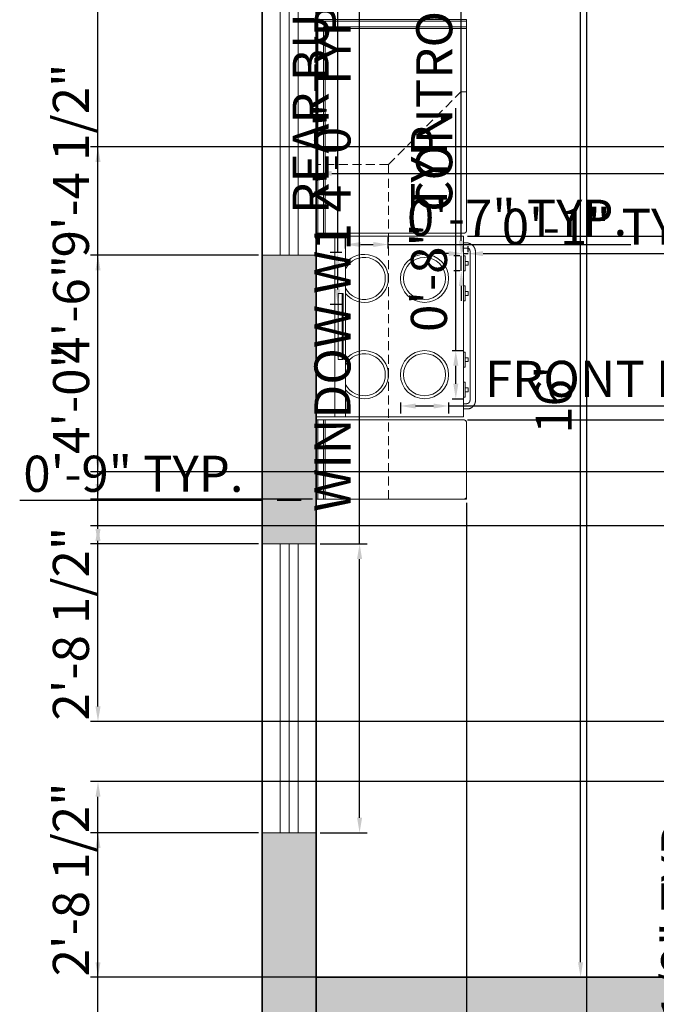
# Model space of a CAD drawing. Units: inches. Extents: x -40 to 424, y -33 to 568.
# Tile 4 of 8: x -40 to 66, y 275 to 438. Entities that reach past the tile are written whole.
import ezdxf

# ---------------------------------------------------------------- set-up
doc = ezdxf.new("R2010")
doc.units = ezdxf.units.IN
doc.linetypes.add('DASHED', pattern=[0.75, 0.5, -0.25])
for name, color, linetype, lineweight in [('A-ANNO-DIMS', 7, 'Continuous', 18), ('A-EQPM', 7, 'Continuous', 13), ('A-FLOR-CASE', 7, 'Continuous', 18), ('A-FLOR-CASE-HIDN', 7, 'DASHED', 13), ('A-GLAZ', 7, 'Continuous', 18), ('A-WALL-PATT', 30, 'Continuous', 13), ('wall', 7, 'Continuous', 35)]:
    doc.layers.add(name, color=color, linetype=linetype, lineweight=lineweight)
doc.styles.get("Standard").update_dxf_attribs({"font": 'arial.ttf'})
doc.dimstyles.new('ISO-25', dxfattribs={"dimtxt": 6, "dimasz": 2.5, "dimexe": 1.25, "dimexo": 0.625, "dimtad": 1, "dimdec": 1, "dimlunit": 3, "dimtxsty": 'Standard', "dimcen": 2.5, "dimadec": 0, "dimazin": 0, "dimtfac": 1, "dimtdec": 1, "dimtmove": 0, "dimatfit": 3, "dimfxl": 1, "dimarcsym": 0})

# ---------------------------------------------------------------- blocks, each defined once
blk = doc.blocks.new('*D27')
at = {"layer": 'A-ANNO-DIMS', "color": 0, "lineweight": -2, "transparency": 16777216}
for p, q in [((52.32, 471), (51.7, 471)), ((52.95, 281.5), (52.95, 468.5)), ((53.57, 279), (54.2, 279))]:
    blk.add_line(p, q, dxfattribs=at)
at = {"layer": 'A-ANNO-DIMS', "color": 0, "transparency": 16777216}
for points in [[(52.53, 468.5), (53.36, 468.5), (52.95, 471)], [(52.53, 281.5), (53.36, 281.5), (52.95, 279)]]:
    blk.add_solid(points, dxfattribs=at)
at = {"layer": 'Defpoints', "color": 0, "transparency": 16777216}
for p in [(52.95, 471), (52.95, 471), (52.95, 279)]:
    blk.add_point(p, dxfattribs=at)
at = {"layer": 'A-ANNO-DIMS', "color": 0, "transparency": 16777216, "insert": (49.26, 375), "char_height": 6, "attachment_point": 5, "rotation": 90}
blk.add_mtext("16'", dxfattribs=at)
blk = doc.blocks.new('*D28')
at = {"layer": 'A-ANNO-DIMS', "color": 0, "lineweight": -2, "transparency": 16777216}
for p, q in [((9.08, 457.74), (9.08, 411.34)), ((165, 457.74), (165, 411.34)), ((11.58, 412.59), (162.5, 412.59))]:
    blk.add_line(p, q, dxfattribs=at)
at = {"layer": 'A-ANNO-DIMS', "color": 0, "transparency": 16777216}
for points in [[(11.58, 413.01), (11.58, 412.18), (9.08, 412.59)], [(162.5, 413.01), (162.5, 412.18), (165, 412.59)]]:
    blk.add_solid(points, dxfattribs=at)
at = {"layer": 'Defpoints', "color": 0, "transparency": 16777216}
for p in [(9.08, 458.36), (165, 458.36), (165, 412.59)]:
    blk.add_point(p, dxfattribs=at)
at = {"layer": 'A-ANNO-DIMS', "color": 0, "transparency": 16777216, "insert": (87.04, 416.28), "char_height": 6, "attachment_point": 5}
blk.add_mtext('12\'-11.9"', dxfattribs=at)
blk = doc.blocks.new('WIN-48IN')
for p, q in [((0, 0), (0, 9)), ((48, 0), (48, 9)), ((0, 6), (48, 6)), ((0, 4.5), (48, 4.5)), ((0, 3), (48, 3))]:
    blk.add_line(p, q)
blk = doc.blocks.new('RANGE-CONTROL')
for p, q in [((0, 2.5), (0.25, 2.5)), ((0, 2.5), (0, 2.46)), ((0, 2.46), (0, 2.33)), ((0, 2.33), (0, 2.13)), ((0, 2.13), (0, 1.87)), ((0, 1.87), (0, 1.57)), ((0.25, 2.46), (0.25, 2.5)), ((0.25, 2.33), (0.25, 2.46)), ((0.25, 2.13), (0.25, 2.33)), ((0.25, 2.13), (0.25, 1.87)), ((0.25, 1.57), (0.25, 1.87)), ((0, 1.57), (0, 1.25)), ((0, 1.25), (0, 0.93)), ((0, 0.93), (0, 0.62)), ((0, 0.62), (0, 0.37)), ((0, 0.37), (0, 0.17)), ((0, 0.17), (0, 0.04)), ((0, 0.04), (0, 0)), ((0.25, 1.57), (0.25, 1.25)), ((0.25, 1.57), (0.75, 1.57)), ((0.25, 1.25), (0.25, 0.93)), ((0.25, 0.93), (0.25, 0.62)), ((0.25, 0.93), (0.75, 0.93)), ((0.25, 0.62), (0.25, 0.37)), ((0.25, 0.37), (0.25, 0.17)), ((0.25, 0.17), (0.25, 0.04)), ((0.25, 0.04), (0.25, 0)), ((0.75, 0.93), (0.75, 1.57)), ((0, 0), (0.25, 0))]:
    blk.add_line(p, q)
blk = doc.blocks.new('RANGE-BURNER-FRONT')
for radius in [4, 3.5]:
    blk.add_circle((4, 4), radius)
blk = doc.blocks.new('RANGE-BURNER-REAR')
for radius, start, end in [(4, 218.9563, 141.0437), (3.5, 207.2878, 152.7122)]:
    blk.add_arc((3.11, 4), radius, start, end)
blk = doc.blocks.new('*D43')
at = {"layer": 'A-ANNO-DIMS', "color": 0, "lineweight": -2, "transparency": 16777216}
for p, q in [((16.2, 351), (16.2, 445.58)), ((9.62, 351), (17.45, 351)), ((16.2, 305.5), (16.2, 348.5)), ((9.62, 303), (17.45, 303))]:
    blk.add_line(p, q, dxfattribs=at)
at = {"layer": 'A-ANNO-DIMS', "color": 0, "transparency": 16777216}
for points in [[(15.78, 348.5), (16.62, 348.5), (16.2, 351)], [(15.78, 305.5), (16.62, 305.5), (16.2, 303)]]:
    blk.add_solid(points, dxfattribs=at)
at = {"layer": 'Defpoints', "color": 0, "transparency": 16777216}
for p in [(9, 351), (16.2, 351), (9, 303)]:
    blk.add_point(p, dxfattribs=at)
at = {"layer": 'A-ANNO-DIMS', "color": 0, "transparency": 16777216, "insert": (12.47, 399.54), "char_height": 6, "attachment_point": 5, "rotation": 90}
blk.add_mtext('WINDOW W1 4\'-0" TYP.', dxfattribs=at)
blk = doc.blocks.new('*D44')
at = {"layer": 'A-ANNO-DIMS', "color": 0, "lineweight": -2, "transparency": 16777216}
for p, q in [((0, 351.62), (0, 359.45)), ((9, 351.62), (9, 359.45)), ((0, 358.2), (-40.32, 358.2)), ((6.5, 358.2), (2.5, 358.2))]:
    blk.add_line(p, q, dxfattribs=at)
at = {"layer": 'A-ANNO-DIMS', "color": 0, "transparency": 16777216}
for points in [[(2.5, 358.62), (2.5, 357.78), (0, 358.2)], [(6.5, 358.62), (6.5, 357.78), (9, 358.2)]]:
    blk.add_solid(points, dxfattribs=at)
at = {"layer": 'Defpoints', "color": 0, "transparency": 16777216}
for p in [(0, 358.2), (0, 351), (9, 351)]:
    blk.add_point(p, dxfattribs=at)
at = {"layer": 'A-ANNO-DIMS', "color": 0, "transparency": 16777216, "insert": (-21.41, 361.89), "char_height": 6, "attachment_point": 5}
blk.add_mtext('0\'-9" TYP.', dxfattribs=at)
blk = doc.blocks.new('*D59')
at = {"layer": 'A-ANNO-DIMS', "color": 0, "lineweight": -2, "transparency": 16777216}
for p, q in [((73.87, 204.92), (73.87, 309.26)), ((83.22, 204.92), (72.62, 204.92)), ((73.87, 140.98), (73.87, 202.42)), ((83.22, 138.48), (72.62, 138.48))]:
    blk.add_line(p, q, dxfattribs=at)
at = {"layer": 'A-ANNO-DIMS', "color": 0, "transparency": 16777216}
for points in [[(73.46, 202.42), (74.29, 202.42), (73.87, 204.92)], [(73.46, 140.98), (74.29, 140.98), (73.87, 138.48)]]:
    blk.add_solid(points, dxfattribs=at)
at = {"layer": 'Defpoints', "color": 0, "transparency": 16777216}
for p in [(73.87, 204.92), (83.84, 204.92), (83.84, 138.48)]:
    blk.add_point(p, dxfattribs=at)
at = {"layer": 'A-ANNO-DIMS', "color": 0, "transparency": 16777216, "insert": (70.14, 258.34), "char_height": 6, "attachment_point": 5, "rotation": 90}
blk.add_mtext('LOW TABLE 5\'-6 1/2" TYP.', dxfattribs=at)
blk = doc.blocks.new('*D71')
at = {"layer": 'A-ANNO-DIMS', "color": 0, "lineweight": -2, "transparency": 16777216}
for p, q in [((33.12, 401.38), (33.12, 498.92)), ((32.88, 398.88), (31.88, 398.88)), ((33.12, 396.38), (33.12, 398.88)), ((32.88, 396.38), (31.88, 396.38)), ((33.12, 393.88), (33.12, 391.38))]:
    blk.add_line(p, q, dxfattribs=at)
at = {"layer": 'A-ANNO-DIMS', "color": 0, "transparency": 16777216}
for points in [[(32.71, 401.38), (33.54, 401.38), (33.12, 398.88)], [(32.71, 393.88), (33.54, 393.88), (33.12, 396.38)]]:
    blk.add_solid(points, dxfattribs=at)
at = {"layer": 'Defpoints', "color": 0, "transparency": 16777216}
for p in [(33.12, 398.88), (33.5, 398.88), (33.5, 396.38)]:
    blk.add_point(p, dxfattribs=at)
at = {"layer": 'A-ANNO-DIMS', "color": 0, "transparency": 16777216, "insert": (29.4, 451.4), "char_height": 6, "attachment_point": 5, "rotation": 90}
blk.add_mtext('CONTROL 0\'-2 1/2" TYP.', dxfattribs=at)
blk = doc.blocks.new('*D72')
at = {"layer": 'A-ANNO-DIMS', "color": 0, "lineweight": -2, "transparency": 16777216}
for p, q in [((31, 399.25), (28.5, 399.25)), ((33.5, 399.5), (33.5, 400.5)), ((33.5, 399.25), (34.25, 399.25)), ((34.25, 399.5), (34.25, 400.5)), ((36.75, 399.25), (77.07, 399.25))]:
    blk.add_line(p, q, dxfattribs=at)
at = {"layer": 'A-ANNO-DIMS', "color": 0, "transparency": 16777216}
for points in [[(31, 399.67), (31, 398.83), (33.5, 399.25)], [(36.75, 399.67), (36.75, 398.83), (34.25, 399.25)]]:
    blk.add_solid(points, dxfattribs=at)
at = {"layer": 'Defpoints', "color": 0, "transparency": 16777216}
for p in [(34.25, 399.25), (33.5, 398.88), (34.25, 398.88)]:
    blk.add_point(p, dxfattribs=at)
at = {"layer": 'A-ANNO-DIMS', "color": 0, "transparency": 16777216, "insert": (58.16, 402.94), "char_height": 6, "attachment_point": 5}
blk.add_mtext('0\'-1" TYP.', dxfattribs=at)
blk = doc.blocks.new('*D73')
at = {"layer": 'A-ANNO-DIMS', "color": 0, "lineweight": -2, "transparency": 16777216}
for p, q in [((23, 374.5), (23, 372.68)), ((25.5, 373.93), (28.5, 373.93)), ((31, 374.5), (31, 372.68)), ((31, 373.93), (139.9, 373.93))]:
    blk.add_line(p, q, dxfattribs=at)
at = {"layer": 'A-ANNO-DIMS', "color": 0, "transparency": 16777216}
for points in [[(25.5, 374.34), (25.5, 373.51), (23, 373.93)], [(28.5, 374.34), (28.5, 373.51), (31, 373.93)]]:
    blk.add_solid(points, dxfattribs=at)
at = {"layer": 'Defpoints', "color": 0, "transparency": 16777216}
for p in [(23, 375.13), (31, 375.13), (31, 373.93)]:
    blk.add_point(p, dxfattribs=at)
at = {"layer": 'A-ANNO-DIMS', "color": 0, "transparency": 16777216, "insert": (86.7, 377.66), "char_height": 6, "attachment_point": 5}
blk.add_mtext('FRONT BURNER 0\'-8" TYP.', dxfattribs=at)
blk = doc.blocks.new('*D74')
at = {"layer": 'A-ANNO-DIMS', "color": 0, "lineweight": -2, "transparency": 16777216}
for p, q in [((32.2, 383.13), (32.2, 423.45)), ((31.62, 383.13), (33.45, 383.13)), ((32.2, 377.63), (32.2, 380.63)), ((31.62, 375.13), (33.45, 375.13))]:
    blk.add_line(p, q, dxfattribs=at)
at = {"layer": 'A-ANNO-DIMS', "color": 0, "transparency": 16777216}
for points in [[(31.78, 380.63), (32.62, 380.63), (32.2, 383.13)], [(31.78, 377.63), (32.62, 377.63), (32.2, 375.13)]]:
    blk.add_solid(points, dxfattribs=at)
at = {"layer": 'Defpoints', "color": 0, "transparency": 16777216}
for p in [(31, 383.13), (32.2, 383.13), (31, 375.13)]:
    blk.add_point(p, dxfattribs=at)
at = {"layer": 'A-ANNO-DIMS', "color": 0, "transparency": 16777216, "insert": (28.51, 404.54), "char_height": 6, "attachment_point": 5, "rotation": 90}
blk.add_mtext('0\'-8" TYP.', dxfattribs=at)
blk = doc.blocks.new('*D75')
at = {"layer": 'A-ANNO-DIMS', "color": 0, "lineweight": -2, "transparency": 16777216}
for p, q in [((12.57, 399.46), (12.57, 516.79)), ((13.25, 399.46), (11.32, 399.46)), ((12.57, 393.29), (12.57, 396.96)), ((13.25, 390.79), (11.32, 390.79))]:
    blk.add_line(p, q, dxfattribs=at)
at = {"layer": 'A-ANNO-DIMS', "color": 0, "transparency": 16777216}
for points in [[(12.15, 396.96), (12.99, 396.96), (12.57, 399.46)], [(12.15, 393.29), (12.99, 393.29), (12.57, 390.79)]]:
    blk.add_solid(points, dxfattribs=at)
at = {"layer": 'Defpoints', "color": 0, "transparency": 16777216}
for p in [(12.57, 399.46), (13.87, 399.46), (13.87, 390.79)]:
    blk.add_point(p, dxfattribs=at)
at = {"layer": 'A-ANNO-DIMS', "color": 0, "transparency": 16777216, "insert": (8.84, 459.38), "char_height": 6, "attachment_point": 5, "rotation": 90}
blk.add_mtext('REAR BURNER 0\'-8 1/2" TYP.', dxfattribs=at)
blk = doc.blocks.new('*D76')
at = {"layer": 'A-ANNO-DIMS', "color": 0, "lineweight": -2, "transparency": 16777216}
for p, q in [((13.87, 400.09), (13.87, 402.01)), ((20.98, 400.09), (20.98, 402.01)), ((16.37, 400.76), (18.48, 400.76)), ((20.98, 400.76), (61.3, 400.76))]:
    blk.add_line(p, q, dxfattribs=at)
at = {"layer": 'A-ANNO-DIMS', "color": 0, "transparency": 16777216}
for points in [[(16.37, 401.18), (16.37, 400.35), (13.87, 400.76)], [(18.48, 401.18), (18.48, 400.35), (20.98, 400.76)]]:
    blk.add_solid(points, dxfattribs=at)
at = {"layer": 'Defpoints', "color": 0, "transparency": 16777216}
for p in [(13.87, 399.46), (20.98, 400.76), (20.98, 399.46)]:
    blk.add_point(p, dxfattribs=at)
at = {"layer": 'A-ANNO-DIMS', "color": 0, "transparency": 16777216, "insert": (42.39, 404.45), "char_height": 6, "attachment_point": 5}
blk.add_mtext('0\'-7" TYP.', dxfattribs=at)
blk = doc.blocks.new('*D83')
at = {"layer": 'A-ANNO-DIMS', "color": 0, "lineweight": -2, "transparency": 16777216}
for p, q in [((-0.63, 303), (-28.55, 303)), ((-27.3, 212.5), (-27.3, 300.5)), ((-0.63, 210), (-28.55, 210))]:
    blk.add_line(p, q, dxfattribs=at)
at = {"layer": 'A-ANNO-DIMS', "color": 0, "transparency": 16777216}
for points in [[(-27.72, 300.5), (-26.88, 300.5), (-27.3, 303)], [(-27.72, 212.5), (-26.88, 212.5), (-27.3, 210)]]:
    blk.add_solid(points, dxfattribs=at)
at = {"layer": 'Defpoints', "color": 0, "transparency": 16777216}
for p in [(-27.3, 303), (0, 303), (0, 210)]:
    blk.add_point(p, dxfattribs=at)
at = {"layer": 'A-ANNO-DIMS', "color": 0, "transparency": 16777216, "insert": (-30.99, 256.5), "char_height": 6, "attachment_point": 5, "rotation": 90}
blk.add_mtext('7\'-9"', dxfattribs=at)
blk = doc.blocks.new('*D84')
at = {"layer": 'A-ANNO-DIMS', "color": 0, "lineweight": -2, "transparency": 16777216}
for p, q in [((-0.63, 399), (-28.55, 399)), ((-27.3, 353.5), (-27.3, 396.5)), ((-0.63, 351), (-28.55, 351))]:
    blk.add_line(p, q, dxfattribs=at)
at = {"layer": 'A-ANNO-DIMS', "color": 0, "transparency": 16777216}
for points in [[(-27.72, 396.5), (-26.88, 396.5), (-27.3, 399)], [(-27.72, 353.5), (-26.88, 353.5), (-27.3, 351)]]:
    blk.add_solid(points, dxfattribs=at)
at = {"layer": 'Defpoints', "color": 0, "transparency": 16777216}
for p in [(-27.3, 399), (0, 399), (0, 351)]:
    blk.add_point(p, dxfattribs=at)
at = {"layer": 'A-ANNO-DIMS', "color": 0, "transparency": 16777216, "insert": (-30.99, 375), "char_height": 6, "attachment_point": 5, "rotation": 90}
blk.add_mtext('4\'-0"', dxfattribs=at)
blk = doc.blocks.new('*D89')
at = {"layer": 'A-ANNO-DIMS', "color": 0, "lineweight": -2, "transparency": 16777216}
for p, q in [((374.38, 417), (-28.55, 417)), ((-27.3, 365.5), (-27.3, 414.5)), ((374.38, 363), (-28.55, 363))]:
    blk.add_line(p, q, dxfattribs=at)
at = {"layer": 'A-ANNO-DIMS', "color": 0, "transparency": 16777216}
for points in [[(-27.72, 414.5), (-26.88, 414.5), (-27.3, 417)], [(-27.72, 365.5), (-26.88, 365.5), (-27.3, 363)]]:
    blk.add_solid(points, dxfattribs=at)
at = {"layer": 'Defpoints', "color": 0, "transparency": 16777216}
for p in [(-27.3, 417), (375, 417), (375, 363)]:
    blk.add_point(p, dxfattribs=at)
at = {"layer": 'A-ANNO-DIMS', "color": 0, "transparency": 16777216, "insert": (-30.99, 390), "char_height": 6, "attachment_point": 5, "rotation": 90}
blk.add_mtext('4\'-6"', dxfattribs=at)
blk = doc.blocks.new('*D91')
at = {"layer": 'A-ANNO-DIMS', "color": 0, "lineweight": -2, "transparency": 16777216}
for p, q in [((9, 90.62), (9, 556.55)), ((54, 90.62), (54, 556.55)), ((11.5, 555.3), (51.5, 555.3))]:
    blk.add_line(p, q, dxfattribs=at)
at = {"layer": 'A-ANNO-DIMS', "color": 0, "transparency": 16777216}
for points in [[(11.5, 555.72), (11.5, 554.88), (9, 555.3)], [(51.5, 555.72), (51.5, 554.88), (54, 555.3)]]:
    blk.add_solid(points, dxfattribs=at)
at = {"layer": 'Defpoints', "color": 0, "transparency": 16777216}
for p in [(54, 555.3), (9, 90), (54, 90)]:
    blk.add_point(p, dxfattribs=at)
at = {"layer": 'A-ANNO-DIMS', "color": 0, "transparency": 16777216, "insert": (31.5, 558.99), "char_height": 6, "attachment_point": 5}
blk.add_mtext('3\'-9"', dxfattribs=at)
blk = doc.blocks.new('*D97')
at = {"layer": 'A-ANNO-DIMS', "color": 0, "lineweight": -2, "transparency": 16777216}
for p, q in [((253.88, 311.5), (-28.55, 311.5)), ((-27.3, 281.5), (-27.3, 309)), ((253.88, 279), (-28.55, 279))]:
    blk.add_line(p, q, dxfattribs=at)
at = {"layer": 'A-ANNO-DIMS', "color": 0, "transparency": 16777216}
for points in [[(-27.72, 309), (-26.88, 309), (-27.3, 311.5)], [(-27.72, 281.5), (-26.88, 281.5), (-27.3, 279)]]:
    blk.add_solid(points, dxfattribs=at)
at = {"layer": 'Defpoints', "color": 0, "transparency": 16777216}
for p in [(-27.3, 311.5), (254.5, 311.5), (254.5, 279)]:
    blk.add_point(p, dxfattribs=at)
at = {"layer": 'A-ANNO-DIMS', "color": 0, "transparency": 16777216, "insert": (-31.03, 295.25), "char_height": 6, "attachment_point": 5, "rotation": 90}
blk.add_mtext('2\'-8 1/2"', dxfattribs=at)
blk = doc.blocks.new('*D99')
at = {"layer": 'A-ANNO-DIMS', "color": 0, "lineweight": -2, "transparency": 16777216}
for p, q in [((244.61, 354), (-28.55, 354)), ((-27.3, 324), (-27.3, 351.5)), ((244.61, 321.5), (-28.55, 321.5))]:
    blk.add_line(p, q, dxfattribs=at)
at = {"layer": 'A-ANNO-DIMS', "color": 0, "transparency": 16777216}
for points in [[(-27.72, 351.5), (-26.88, 351.5), (-27.3, 354)], [(-27.72, 324), (-26.88, 324), (-27.3, 321.5)]]:
    blk.add_solid(points, dxfattribs=at)
at = {"layer": 'Defpoints', "color": 0, "transparency": 16777216}
for p in [(-27.3, 354), (245.23, 354), (245.23, 321.5)]:
    blk.add_point(p, dxfattribs=at)
at = {"layer": 'A-ANNO-DIMS', "color": 0, "transparency": 16777216, "insert": (-31.03, 337.75), "char_height": 6, "attachment_point": 5, "rotation": 90}
blk.add_mtext('2\'-8 1/2"', dxfattribs=at)
blk = doc.blocks.new('*D100')
at = {"layer": 'A-ANNO-DIMS', "color": 0, "lineweight": -2, "transparency": 16777216}
for p, q in [((8.37, 471), (-28.55, 471)), ((-27.3, 360.94), (-27.3, 468.5)), ((8.37, 358.44), (-28.55, 358.44))]:
    blk.add_line(p, q, dxfattribs=at)
at = {"layer": 'A-ANNO-DIMS', "color": 0, "transparency": 16777216}
for points in [[(-27.72, 468.5), (-26.88, 468.5), (-27.3, 471)], [(-27.72, 360.94), (-26.88, 360.94), (-27.3, 358.44)]]:
    blk.add_solid(points, dxfattribs=at)
at = {"layer": 'Defpoints', "color": 0, "transparency": 16777216}
for p in [(-27.3, 471), (9, 471), (9, 358.44)]:
    blk.add_point(p, dxfattribs=at)
at = {"layer": 'A-ANNO-DIMS', "color": 0, "transparency": 16777216, "insert": (-31.03, 414.72), "char_height": 6, "attachment_point": 5, "rotation": 90}
blk.add_mtext('9\'-4 1/2"', dxfattribs=at)
blk = doc.blocks.new('*D101')
at = {"layer": 'A-ANNO-DIMS', "color": 0, "lineweight": -2, "transparency": 16777216}
for p, q in [((9, 357.82), (9, -28.55)), ((34, 357.82), (34, -28.55)), ((11.5, -27.3), (31.5, -27.3))]:
    blk.add_line(p, q, dxfattribs=at)
at = {"layer": 'A-ANNO-DIMS', "color": 0, "transparency": 16777216}
for points in [[(11.5, -26.88), (11.5, -27.72), (9, -27.3)], [(31.5, -26.88), (31.5, -27.72), (34, -27.3)]]:
    blk.add_solid(points, dxfattribs=at)
at = {"layer": 'Defpoints', "color": 0, "transparency": 16777216}
for p in [(9, 358.44), (34, 358.44), (34, -27.3)]:
    blk.add_point(p, dxfattribs=at)
at = {"layer": 'A-ANNO-DIMS', "color": 0, "transparency": 16777216, "insert": (21.5, -23.66), "char_height": 6, "attachment_point": 5}
blk.add_mtext('2\'-1"', dxfattribs=at)
blk = doc.blocks.new('*D103')
at = {"layer": 'A-ANNO-DIMS', "color": 0, "lineweight": -2, "transparency": 16777216}
for p, q in [((411.3, 402.13), (411.3, 435.91)), ((34.13, 402.13), (412.55, 402.13)), ((411.3, 374.13), (411.3, 399.63)), ((34.13, 371.63), (412.55, 371.63))]:
    blk.add_line(p, q, dxfattribs=at)
at = {"layer": 'A-ANNO-DIMS', "color": 0, "transparency": 16777216}
for points in [[(410.88, 399.63), (411.72, 399.63), (411.3, 402.13)], [(410.88, 374.13), (411.72, 374.13), (411.3, 371.63)]]:
    blk.add_solid(points, dxfattribs=at)
at = {"layer": 'Defpoints', "color": 0, "transparency": 16777216}
for p in [(33.5, 402.13), (411.3, 402.13), (33.5, 371.63)]:
    blk.add_point(p, dxfattribs=at)
at = {"layer": 'A-ANNO-DIMS', "color": 0, "transparency": 16777216, "insert": (407.57, 420.27), "char_height": 6, "attachment_point": 5, "rotation": 90}
blk.add_mtext('2\'-6 1/2"', dxfattribs=at)

msp = doc.modelspace()

# ---------------------------------------------------------------- hatches: boundary and pattern name
at = {"layer": 'A-WALL-PATT'}
h = msp.add_hatch(color=256, dxfattribs=at)
h.dxf.hatch_style = 1
h.paths.add_polyline_path([(9, 399), (0, 399), (0, 351), (9, 351)])
h.paths.add_polyline_path([(9, 303), (0, 303), (0, 210), (9, 210)])
h.paths.add_polyline_path([(9, 150), (0, 150), (0, 0), (384, 0), (384, 69), (375, 69), (375, 62.24), (375, 9), (9, 9)])
h.paths.add_polyline_path([(210, 177), (216, 177), (216, 186), (210, 186), (210, 216), (201, 216), (201, 90), (195, 90), (195, 81), (201, 81), (201, 9), (210, 9)])
h.paths.add_polyline_path([(384, 216), (375, 216), (375, 117), (384, 117)])
h.paths.add_polyline_path([(384, 298.5), (375, 298.5), (375, 279), (375, 240), (384, 240)])
h.paths.add_polyline_path([(384, 417), (375, 417), (375, 334.5), (384, 334.5)])
h.paths.add_polyline_path([(384, 528), (216, 528), (216, 519), (375, 519), (375, 465), (384, 465)])
h.paths.add_polyline_path([(192, 528), (0, 528), (0, 511.5), (9, 511.5), (9, 519), (192, 519)])
h.paths.add_polyline_path([(9, 487.5), (0, 487.5), (0, 447), (9, 447)])
h.paths.add_polyline_path([(111, 480), (9, 480), (9, 471), (111, 471)])
h.paths.add_polyline_path([(174, 519), (165, 519), (165, 354), (174, 354)])
h.paths.add_polyline_path([(243, 426), (237.86, 426), (234, 426), (234, 420), (174, 420), (174, 411), (234, 411), (234, 405), (239.14, 405), (243, 405)])
h.paths.add_polyline_path([(243, 519), (234, 519), (234, 460.14, -0.031638), (237.86, 460.2), (237.86, 462), (243, 462)])
h.paths.add_polyline_path([(243, 369), (234, 369), (234, 354), (375, 354), (375, 363), (243, 363)])
h.paths.add_polyline_path([(375, 279), (195, 279), (195, 270), (201, 270), (201, 264), (210, 264), (210, 270), (375, 270)])
h.paths.add_polyline_path([(291, 270), (282, 270), (282, 222), (286.29, 222), (291, 222)])
h.paths.add_polyline_path([(375, 186), (291, 186), (291, 192), (282, 192), (282, 186), (252, 186), (252, 180.86), (252, 177), (375, 177)])
h.paths.add_polyline_path([(147, 279), (9, 279), (9, 270), (147, 270)])

# ---------------------------------------------------------------- linework, layer by layer
at = {"layer": 'A-EQPM'}
for p, q in [((9, 372.13), (9, 402.13)), ((11.52, 402.13), (9, 402.13)), ((11.52, 402.13), (11.58, 402.13)), ((11.58, 402.13), (11.63, 402.13)), ((11.63, 402.13), (11.64, 402.13)), ((11.64, 402.13), (11.65, 402.13)), ((11.65, 402.13), (11.66, 402.13)), ((11.66, 402.13), (11.68, 402.13)), ((11.68, 402.13), (11.69, 402.13)), ((11.69, 402.13), (11.74, 402.13)), ((11.74, 402.13), (11.79, 402.13)), ((11.79, 402.13), (11.84, 402.13)), ((11.84, 402.13), (11.89, 402.13)), ((11.89, 402.13), (11.93, 402.13)), ((11.93, 402.13), (11.98, 402.13)), ((11.98, 402.13), (12.02, 402.13)), ((12.02, 402.13), (12.06, 402.13)), ((12.06, 402.13), (12.09, 402.13)), ((12.09, 372.13), (12.09, 402.13)), ((12.09, 402.13), (13.83, 402.13)), ((13.83, 402.13), (13.85, 402.13)), ((13.86, 402.13), (13.85, 402.13)), ((13.85, 402.13), (13.85, 402.13)), ((13.86, 402.13), (13.86, 402.13)), ((13.86, 402.13), (13.87, 402.13)), ((13.87, 402.13), (13.87, 402.13)), ((13.87, 402.13), (13.87, 402.13)), ((13.87, 397.56), (13.87, 402.13)), ((13.87, 402.13), (32.84, 402.13)), ((32.84, 402.13), (32.91, 402.13)), ((32.91, 402.13), (32.98, 402.13)), ((32.98, 402.13), (33.05, 402.13)), ((33.05, 402.13), (33.12, 402.13)), ((33.12, 402.13), (33.13, 402.13)), ((33.13, 402.13), (33.18, 402.13)), ((33.18, 402.13), (33.24, 402.13)), ((33.24, 402.13), (33.3, 402.13)), ((33.3, 402.13), (33.35, 402.13)), ((33.35, 402.13), (33.36, 402.13)), ((33.36, 402.13), (33.4, 402.13)), ((33.4, 402.13), (33.44, 402.13)), ((33.44, 402.13), (33.46, 402.13)), ((33.46, 402.13), (33.47, 402.13)), ((33.47, 402.13), (33.5, 402.13)), ((33.5, 402.13), (33.5, 401.05)), ((33.5, 401.05), (33.97, 401.05)), ((33.5, 401.05), (33.5, 400.98)), ((33.5, 400.98), (33.5, 400.97)), ((33.5, 400.97), (33.5, 400.9)), ((33.5, 400.9), (33.5, 400.78)), ((33.5, 400.78), (33.5, 400.62)), ((33.5, 400.62), (33.5, 400.45)), ((33.5, 400.45), (33.5, 400.31)), ((33.5, 400.31), (33.5, 400.21)), ((33.5, 400.21), (33.5, 400.18)), ((34.08, 400.18), (33.5, 400.18)), ((33.5, 400.18), (33.5, 398.88)), ((34.57, 399.66), (34.57, 374.91)), ((35.47, 399.58), (35.47, 374.83)), ((13.87, 381.64), (13.87, 397.56)), ((33.5, 396.38), (33.5, 393.88)), ((12.63, 381.63), (12.63, 392.63)), ((12.63, 392.63), (13.31, 392.63)), ((13.31, 392.63), (13.31, 381.63)), ((13.31, 392.63), (13.49, 392.63)), ((13.49, 392.63), (13.49, 381.63)), ((33.5, 391.38), (33.5, 382.88)), ((13.31, 381.63), (12.63, 381.63)), ((13.49, 381.63), (13.31, 381.63)), ((13.87, 376.61), (13.87, 381.64)), ((33.5, 380.38), (33.5, 377.88)), ((13.87, 372.13), (13.87, 376.61)), ((33.5, 375.38), (33.5, 374.31)), ((33.97, 374.31), (33.5, 374.31)), ((33.5, 374.31), (33.5, 374.27)), ((33.5, 374.27), (33.5, 374.23)), ((33.5, 374.23), (33.5, 374.19)), ((33.5, 374.19), (33.5, 374.09)), ((33.5, 374.09), (33.5, 373.95)), ((33.5, 373.95), (33.5, 373.78)), ((33.5, 373.78), (33.5, 373.63)), ((33.5, 373.63), (33.5, 373.5)), ((33.5, 373.5), (33.5, 373.43)), ((34.08, 373.43), (33.5, 373.43)), ((33.5, 373.43), (33.5, 372.13)), ((11.52, 372.13), (9, 372.13)), ((11.52, 372.13), (11.58, 372.13)), ((11.63, 372.13), (11.58, 372.13)), ((11.64, 372.13), (11.63, 372.13)), ((11.65, 372.13), (11.64, 372.13)), ((11.65, 372.13), (11.66, 372.13)), ((11.66, 372.13), (11.68, 372.13)), ((11.68, 372.13), (11.69, 372.13)), ((11.69, 372.13), (11.74, 372.13)), ((11.74, 372.13), (11.79, 372.13)), ((11.79, 372.13), (11.84, 372.13)), ((11.84, 372.13), (11.89, 372.13)), ((11.89, 372.13), (11.93, 372.13)), ((11.93, 372.13), (11.98, 372.13)), ((11.98, 372.13), (12.02, 372.13)), ((12.02, 372.13), (12.06, 372.13)), ((12.06, 372.13), (12.09, 372.13)), ((13.83, 372.13), (12.09, 372.13)), ((13.83, 372.13), (13.85, 372.13)), ((13.85, 372.13), (13.85, 372.13)), ((13.85, 372.13), (13.86, 372.13)), ((13.86, 372.13), (13.86, 372.13)), ((13.86, 372.13), (13.87, 372.13)), ((13.87, 372.13), (13.87, 372.13)), ((13.87, 372.13), (13.87, 372.13)), ((32.84, 372.13), (13.87, 372.13)), ((32.84, 372.13), (32.91, 372.13)), ((32.91, 372.13), (32.98, 372.13)), ((32.98, 372.13), (32.99, 372.13)), ((32.98, 372.13), (32.99, 372.13)), ((32.98, 372.13), (32.98, 372.13)), ((32.99, 372.13), (33.05, 372.13)), ((33.05, 372.13), (33.12, 372.13)), ((33.12, 372.13), (33.13, 372.13)), ((33.13, 372.13), (33.18, 372.13)), ((33.18, 372.13), (33.24, 372.13)), ((33.24, 372.13), (33.3, 372.13)), ((33.3, 372.13), (33.35, 372.13)), ((33.35, 372.13), (33.36, 372.13)), ((33.36, 372.13), (33.4, 372.13)), ((33.44, 372.13), (33.4, 372.13)), ((33.44, 372.13), (33.46, 372.13)), ((33.46, 372.13), (33.47, 372.13)), ((33.5, 372.13), (33.47, 372.13))]:
    msp.add_line(p, q, dxfattribs=at)
for points in [[(33.97, 401.05), (34.05, 401.04), (34.12, 401.03), (34.17, 401.02), (34.23, 401.02), (34.27, 401.01), (34.31, 401), (34.35, 400.99), (34.38, 400.98), (34.41, 400.97), (34.44, 400.96), (34.47, 400.95), (34.5, 400.94), (34.53, 400.93), (34.55, 400.91), (34.58, 400.9), (34.6, 400.89), (34.62, 400.88), (34.65, 400.86), (34.67, 400.85), (34.69, 400.84), (34.71, 400.83), (34.73, 400.81), (34.75, 400.8), (34.77, 400.79), (34.78, 400.78), (34.79, 400.77), (34.8, 400.77), (34.81, 400.76), (34.82, 400.75), (34.83, 400.75), (34.84, 400.74), (34.84, 400.74), (34.85, 400.73), (34.86, 400.73), (34.86, 400.72), (34.87, 400.72), (34.88, 400.71), (34.89, 400.7), (34.9, 400.69), (34.92, 400.68), (34.93, 400.67), (34.95, 400.66), (34.97, 400.64), (34.98, 400.63), (35, 400.61), (35.02, 400.59), (35.04, 400.57), (35.06, 400.56), (35.08, 400.54), (35.1, 400.52), (35.12, 400.5), (35.13, 400.48), (35.15, 400.45), (35.17, 400.43), (35.19, 400.41), (35.2, 400.39), (35.22, 400.37), (35.23, 400.35), (35.25, 400.32), (35.26, 400.3), (35.28, 400.28), (35.29, 400.25), (35.3, 400.23), (35.32, 400.2), (35.33, 400.18), (35.34, 400.16), (35.35, 400.13), (35.36, 400.1), (35.37, 400.08), (35.38, 400.05), (35.39, 400.02), (35.4, 399.99), (35.41, 399.95), (35.42, 399.92), (35.43, 399.88), (35.44, 399.83), (35.45, 399.78), (35.46, 399.72), (35.47, 399.65), (35.47, 399.58)], [(34.08, 400.18), (34.11, 400.17), (34.14, 400.17), (34.17, 400.17), (34.19, 400.16), (34.21, 400.16), (34.23, 400.15), (34.24, 400.15), (34.26, 400.15), (34.27, 400.14), (34.28, 400.14), (34.3, 400.13), (34.31, 400.13), (34.32, 400.12), (34.33, 400.12), (34.34, 400.12), (34.34, 400.11), (34.35, 400.11), (34.36, 400.11), (34.36, 400.11), (34.36, 400.1), (34.37, 400.1), (34.37, 400.1), (34.37, 400.1), (34.38, 400.1), (34.38, 400.09), (34.38, 400.09), (34.38, 400.09), (34.39, 400.09), (34.39, 400.08), (34.39, 400.08), (34.4, 400.08), (34.4, 400.07), (34.41, 400.06), (34.41, 400.06), (34.42, 400.05), (34.43, 400.04), (34.43, 400.03), (34.44, 400.03), (34.45, 400.02), (34.46, 400.01), (34.46, 400), (34.47, 399.99), (34.47, 399.98), (34.48, 399.97), (34.49, 399.96), (34.49, 399.95), (34.5, 399.94), (34.5, 399.93), (34.51, 399.92), (34.51, 399.91), (34.52, 399.89), (34.52, 399.88), (34.53, 399.87), (34.53, 399.86), (34.54, 399.85), (34.54, 399.83), (34.55, 399.82), (34.55, 399.8), (34.55, 399.78), (34.56, 399.77), (34.56, 399.74), (34.57, 399.72), (34.57, 399.69), (34.57, 399.66)], [(34.57, 374.91), (34.57, 374.87), (34.57, 374.84), (34.56, 374.82), (34.56, 374.8), (34.55, 374.78), (34.55, 374.76), (34.55, 374.74), (34.54, 374.73), (34.54, 374.71), (34.53, 374.7), (34.53, 374.69), (34.52, 374.68), (34.52, 374.67), (34.51, 374.66), (34.51, 374.64), (34.5, 374.63), (34.5, 374.62), (34.49, 374.61), (34.49, 374.6), (34.48, 374.59), (34.47, 374.58), (34.47, 374.57), (34.46, 374.56), (34.46, 374.55), (34.45, 374.54), (34.44, 374.54), (34.43, 374.53), (34.43, 374.52), (34.42, 374.51), (34.41, 374.5), (34.4, 374.49), (34.39, 374.48), (34.39, 374.47), (34.38, 374.47), (34.37, 374.46), (34.36, 374.45), (34.35, 374.44), (34.34, 374.44), (34.33, 374.43), (34.32, 374.42), (34.31, 374.42), (34.3, 374.41), (34.29, 374.4), (34.28, 374.4), (34.27, 374.39), (34.26, 374.38), (34.25, 374.38), (34.24, 374.37), (34.23, 374.37), (34.22, 374.36), (34.21, 374.36), (34.2, 374.35), (34.19, 374.35), (34.18, 374.34), (34.16, 374.34), (34.15, 374.34), (34.13, 374.33), (34.12, 374.33), (34.1, 374.32), (34.08, 374.32), (34.06, 374.32), (34.03, 374.31), (34, 374.31), (33.97, 374.31)], [(35.47, 374.83), (35.47, 374.75), (35.46, 374.68), (35.45, 374.62), (35.44, 374.57), (35.43, 374.53), (35.42, 374.49), (35.41, 374.45), (35.4, 374.41), (35.39, 374.38), (35.38, 374.35), (35.37, 374.32), (35.36, 374.3), (35.35, 374.27), (35.34, 374.25), (35.33, 374.22), (35.32, 374.2), (35.3, 374.17), (35.29, 374.15), (35.28, 374.12), (35.26, 374.1), (35.25, 374.08), (35.23, 374.06), (35.22, 374.03), (35.2, 374.01), (35.19, 373.99), (35.17, 373.97), (35.15, 373.95), (35.13, 373.93), (35.12, 373.91), (35.1, 373.88), (35.08, 373.87), (35.06, 373.85), (35.04, 373.83), (35.02, 373.81), (35, 373.79), (34.98, 373.77), (34.96, 373.75), (34.94, 373.74), (34.92, 373.72), (34.9, 373.7), (34.87, 373.69), (34.85, 373.67), (34.83, 373.66), (34.81, 373.64), (34.78, 373.63), (34.76, 373.62), (34.73, 373.6), (34.71, 373.59), (34.69, 373.58), (34.66, 373.57), (34.64, 373.56), (34.61, 373.54), (34.58, 373.53), (34.55, 373.52), (34.52, 373.51), (34.49, 373.5), (34.46, 373.49), (34.42, 373.48), (34.38, 373.47), (34.34, 373.47), (34.28, 373.46), (34.23, 373.45), (34.16, 373.44), (34.08, 373.43)]]:
    msp.add_lwpolyline(points, dxfattribs=at)
at = {"layer": 'A-FLOR-CASE'}
for p, q in [((9, 438.13), (9.25, 438.13)), ((9, 402.63), (9, 438.13)), ((34, 438.13), (9.25, 438.13)), ((9.25, 402.63), (9.25, 437.88)), ((34, 437.88), (9.25, 437.88)), ((16.61, 436.94), (10.19, 436.94)), ((10.19, 430.52), (10.19, 436.94)), ((34, 436.94), (16.61, 436.94)), ((34, 438.13), (34, 403.13)), ((10.46, 402.63), (10.46, 436.66)), ((16.33, 436.66), (10.46, 436.66)), ((34, 436.66), (16.33, 436.66)), ((10.19, 402.63), (10.19, 430.52)), ((9, 402.63), (9.25, 402.63)), ((9.25, 402.63), (9.38, 402.63)), ((9.38, 402.63), (9.5, 402.63)), ((9.5, 402.63), (9.61, 402.63)), ((9.61, 402.63), (9.72, 402.63)), ((9.72, 402.63), (9.81, 402.63)), ((9.81, 402.63), (9.9, 402.63)), ((9.9, 402.63), (9.97, 402.63)), ((9.97, 402.63), (10.04, 402.63)), ((10.04, 402.63), (10.09, 402.63)), ((10.09, 402.63), (10.11, 402.63)), ((10.11, 402.63), (10.13, 402.63)), ((10.13, 402.63), (10.16, 402.63)), ((10.16, 402.63), (10.18, 402.63)), ((10.18, 402.63), (10.19, 402.63)), ((10.19, 402.63), (10.21, 402.63)), ((10.21, 402.63), (10.24, 402.63)), ((10.24, 402.63), (10.27, 402.63)), ((10.27, 402.63), (10.31, 402.63)), ((10.31, 402.63), (10.34, 402.63)), ((10.34, 402.63), (10.38, 402.63)), ((10.38, 402.63), (10.42, 402.63)), ((10.42, 402.63), (10.46, 402.63)), ((10.46, 402.63), (33.5, 402.63)), ((33.5, 402.63), (33.53, 402.63)), ((33.53, 402.63), (33.57, 402.63)), ((33.57, 402.63), (33.6, 402.64)), ((33.6, 402.64), (33.63, 402.64)), ((33.63, 402.64), (33.66, 402.65)), ((33.66, 402.65), (33.69, 402.66)), ((33.69, 402.66), (33.72, 402.68)), ((33.72, 402.68), (33.75, 402.69)), ((33.75, 402.69), (33.78, 402.71)), ((33.78, 402.71), (33.8, 402.73)), ((33.8, 402.73), (33.83, 402.75)), ((33.83, 402.75), (33.85, 402.77)), ((33.85, 402.77), (33.88, 402.8)), ((33.88, 402.8), (33.9, 402.82)), ((33.9, 402.82), (33.92, 402.85)), ((33.92, 402.85), (33.93, 402.88)), ((33.93, 402.88), (33.95, 402.9)), ((33.95, 402.9), (33.96, 402.93)), ((33.96, 402.93), (33.97, 402.96)), ((33.97, 402.96), (33.98, 403)), ((33.98, 403), (33.99, 403.03)), ((33.99, 403.03), (34, 403.06)), ((34, 403.13), (34, 403.12)), ((34, 403.12), (34, 403.12)), ((34, 403.12), (34, 403.09)), ((34, 403.06), (34, 403.09)), ((9.25, 371.63), (9, 371.63)), ((9, 371.63), (9, 359.63)), ((9.25, 371.63), (9.38, 371.63)), ((9.25, 358.44), (9.25, 371.63)), ((9.38, 371.63), (9.5, 371.63)), ((9.5, 371.63), (9.61, 371.63)), ((9.61, 371.63), (9.72, 371.63)), ((9.72, 371.63), (9.81, 371.63)), ((9.81, 371.63), (9.9, 371.63)), ((9.9, 371.63), (9.97, 371.63)), ((9.97, 371.63), (10.04, 371.63)), ((10.04, 371.63), (10.09, 371.63)), ((10.09, 371.63), (10.11, 371.63)), ((10.11, 371.63), (10.13, 371.63)), ((10.13, 371.63), (10.16, 371.63)), ((10.16, 371.63), (10.18, 371.63)), ((10.18, 371.63), (10.19, 371.63)), ((10.19, 371.63), (10.21, 371.63)), ((10.19, 359.63), (10.19, 371.63)), ((10.21, 371.63), (10.24, 371.63)), ((10.24, 371.63), (10.27, 371.63)), ((10.27, 371.63), (10.31, 371.63)), ((10.31, 371.63), (10.34, 371.63)), ((10.34, 371.63), (10.38, 371.63)), ((10.38, 371.63), (10.42, 371.63)), ((10.42, 371.63), (10.46, 371.63)), ((10.46, 358.44), (10.46, 371.63)), ((33.5, 371.63), (10.46, 371.63)), ((33.5, 371.63), (33.53, 371.62)), ((33.53, 371.62), (33.57, 371.62)), ((33.57, 371.62), (33.6, 371.62)), ((33.6, 371.62), (33.63, 371.61)), ((33.63, 371.61), (33.66, 371.6)), ((33.66, 371.6), (33.69, 371.59)), ((33.69, 371.59), (33.72, 371.57)), ((33.72, 371.57), (33.75, 371.56)), ((33.75, 371.56), (33.78, 371.54)), ((33.78, 371.54), (33.8, 371.52)), ((33.8, 371.52), (33.83, 371.5)), ((33.83, 371.5), (33.85, 371.48)), ((33.85, 371.48), (33.88, 371.46)), ((33.88, 371.46), (33.9, 371.43)), ((33.9, 371.43), (33.92, 371.4)), ((33.92, 371.4), (33.93, 371.38)), ((33.93, 371.38), (33.95, 371.35)), ((33.95, 371.35), (33.96, 371.32)), ((33.96, 371.32), (33.97, 371.29)), ((33.97, 371.29), (33.98, 371.26)), ((33.98, 371.26), (33.99, 371.22)), ((33.99, 371.22), (34, 371.19)), ((34, 371.19), (34, 371.16)), ((34, 371.16), (34, 371.13)), ((34, 358.94), (34, 371.13)), ((9, 359.63), (9, 359.63)), ((9, 359.63), (9, 358.44)), ((9, 358.44), (9, 358.44)), ((9, 358.44), (9.25, 358.44)), ((9.25, 358.44), (9.38, 358.44)), ((9.38, 358.44), (9.5, 358.44)), ((9.5, 358.44), (9.61, 358.44)), ((9.61, 358.44), (9.72, 358.44)), ((9.72, 358.44), (9.81, 358.44)), ((9.81, 358.44), (9.9, 358.44)), ((9.9, 358.44), (9.97, 358.44)), ((9.97, 358.44), (10.04, 358.44)), ((10.04, 358.44), (10.09, 358.44)), ((10.09, 359.63), (10.11, 359.63)), ((10.09, 359.63), (10.11, 359.63)), ((10.09, 358.44), (10.11, 358.44)), ((10.09, 358.44), (10.11, 358.44)), ((10.11, 359.63), (10.13, 359.63)), ((10.11, 359.63), (10.13, 359.63)), ((10.11, 358.44), (10.13, 358.44)), ((10.11, 358.44), (10.13, 358.44)), ((10.13, 358.44), (10.16, 358.44)), ((10.16, 359.63), (10.18, 359.63)), ((10.16, 359.63), (10.18, 359.63)), ((10.16, 358.44), (10.18, 358.44)), ((10.16, 358.44), (10.18, 358.44)), ((10.18, 359.63), (10.19, 359.63)), ((10.18, 359.63), (10.19, 359.63)), ((10.18, 358.44), (10.19, 358.44)), ((10.18, 358.44), (10.19, 358.44)), ((10.19, 359.63), (10.21, 359.63)), ((10.19, 359.63), (10.21, 359.63)), ((10.19, 358.44), (10.19, 359.63)), ((10.19, 359.63), (10.19, 359.63)), ((10.19, 358.44), (10.21, 358.44)), ((10.19, 358.44), (10.19, 358.44)), ((10.19, 358.44), (10.21, 358.44)), ((10.21, 358.44), (10.24, 358.44)), ((10.24, 359.63), (10.27, 359.63)), ((10.24, 359.63), (10.27, 359.63)), ((10.24, 358.44), (10.27, 358.44)), ((10.24, 358.44), (10.27, 358.44)), ((10.27, 358.44), (10.31, 358.44)), ((10.31, 359.63), (10.34, 359.63)), ((10.31, 359.63), (10.34, 359.63)), ((10.31, 358.44), (10.34, 358.44)), ((10.34, 358.44), (10.31, 358.44)), ((10.34, 358.44), (10.38, 358.44)), ((10.34, 358.44), (10.34, 358.44)), ((10.38, 359.63), (10.42, 359.63)), ((10.38, 359.63), (10.42, 359.63)), ((10.38, 358.44), (10.42, 358.44)), ((10.38, 358.44), (10.42, 358.44)), ((10.42, 358.44), (10.46, 358.44)), ((33.5, 358.44), (10.46, 358.44)), ((33.5, 358.44), (33.53, 358.44)), ((33.53, 358.44), (33.57, 358.44)), ((33.53, 358.44), (34, 358.44)), ((33.57, 358.44), (33.6, 358.45)), ((33.57, 358.44), (33.57, 358.44)), ((33.57, 358.44), (34, 358.44)), ((33.6, 358.45), (33.63, 358.46)), ((33.63, 358.46), (33.66, 358.46)), ((33.66, 358.46), (33.69, 358.48)), ((33.69, 358.48), (33.72, 358.49)), ((33.72, 358.49), (33.75, 358.51)), ((33.75, 358.51), (33.78, 358.52)), ((33.78, 358.52), (33.8, 358.54)), ((33.8, 358.54), (33.83, 358.56)), ((33.83, 358.56), (33.85, 358.58)), ((33.85, 358.58), (33.88, 358.61)), ((33.88, 358.61), (33.9, 358.63)), ((33.9, 358.63), (33.92, 358.66)), ((33.92, 358.66), (33.93, 358.69)), ((33.93, 358.69), (33.95, 358.72)), ((33.95, 358.72), (33.96, 358.75)), ((33.96, 358.75), (33.97, 358.78)), ((33.97, 358.78), (33.98, 358.81)), ((33.98, 358.81), (33.99, 358.84)), ((33.99, 358.84), (34, 358.87)), ((34, 358.91), (34, 358.94)), ((34, 358.87), (34, 358.91)), ((34, 358.44), (34, 358.91)), ((34, 358.44), (34, 358.44))]:
    msp.add_line(p, q, dxfattribs=at)
at = {"layer": 'A-FLOR-CASE-HIDN', "ltscale": 3}
msp.add_line((21, 414.04), (33.02, 426.13), dxfattribs=at)
msp.add_lwpolyline([(34, 438.13), (33.02, 438.13), (33.02, 426.13), (34, 426.13)], dxfattribs=at)
msp.add_lwpolyline([(9, 358.44), (21, 358.44), (21, 414.04), (9, 414.04)], close=True, dxfattribs=at)
at = {"layer": 'wall'}
for p, q in [((9, 519), (9, 9)), ((9, 279), (147, 279))]:
    msp.add_line(p, q, dxfattribs=at)
msp.add_lwpolyline([(0, 0), (384, 0), (384, 528), (0, 528)], close=True, dxfattribs=at)

# ---------------------------------------------------------------- block references
at = {"layer": 'A-EQPM'}
for name, p in [('RANGE-BURNER-REAR', (13.87, 391.13)), ('RANGE-BURNER-FRONT', (23, 391.13)), ('RANGE-CONTROL', (33.5, 396.38)), ('RANGE-CONTROL', (33.5, 391.38)), ('RANGE-BURNER-REAR', (13.87, 375.13)), ('RANGE-BURNER-FRONT', (23, 375.13)), ('RANGE-CONTROL', (33.5, 380.38)), ('RANGE-CONTROL', (33.5, 375.38))]:
    msp.add_blockref(name, p, dxfattribs=at)
at = {"layer": 'A-GLAZ', "rotation": 90.00000000000003}
for p in [(9, 399), (9, 303)]:
    msp.add_blockref('WIN-48IN', p, dxfattribs=at)

# ---------------------------------------------------------------- dimensions: what is measured, and where the dimension line sits
at = {"layer": 'A-ANNO-DIMS'}
for base, p1, p2, override, picture, middle in [((54, 555.3), (9, 90), (54, 90), {"dimdec": 1, "dimlfac": 1, "dimrnd": 0, "dimzin": 1, "dimdsep": 46, "dimlunit": 4, "dimfrac": 2}, '*D91', (31.5, 558.99)), ((165, 412.59), (9.08, 458.36), (165, 458.36), {"dimclrd": 0, "dimclre": 0, "dimclrt": 0}, '*D28', (87.04, 416.28)), ((34, -27.3), (9, 358.44), (34, 358.44), {"dimdec": 1, "dimlfac": 1, "dimrnd": 0, "dimzin": 1, "dimdsep": 46, "dimlunit": 4, "dimfrac": 2}, '*D101', (21.5, -23.66))]:
    dim = msp.add_linear_dim(base=base, p1=p1, p2=p2, dimstyle='ISO-25', override=override, dxfattribs=at)
    dim.commit()
    dim.dimension.update_dxf_attribs({"geometry": picture, "text_midpoint": middle})
for base, p1, p2, angle, text, picture, middle in [((12.57, 399.46), (13.87, 390.79), (13.87, 399.46), 90, 'REAR BURNER <> TYP.', '*D75', (8.84, 459.38)), ((33.13, 398.88), (33.5, 396.38), (33.5, 398.88), 90, 'CONTROL <> TYP.', '*D71', (29.4, 451.4)), ((16.2, 351), (9, 303), (9, 351), 90, 'WINDOW W1 <> TYP.', '*D43', (12.47, 399.54)), ((32.2, 383.13), (31, 375.13), (31, 383.13), 90, '<> TYP.', '*D74', (28.51, 404.54)), ((0, 358.2), (9, 351), (0, 351), 180, '<> TYP.', '*D44', (-21.41, 361.89)), ((73.87, 204.92), (83.84, 138.48), (83.84, 204.92), 90, 'LOW TABLE <> TYP.', '*D59', (70.14, 258.34))]:
    dim = msp.add_linear_dim(base=base, p1=p1, p2=p2, angle=angle, text=text, dimstyle='ISO-25', override={"dimdec": 1, "dimlfac": 1, "dimrnd": 0, "dimzin": 1, "dimdsep": 46, "dimlunit": 4, "dimfrac": 2}, dxfattribs=at)
    dim.commit()
    dim.dimension.update_dxf_attribs({"geometry": picture, "text_midpoint": middle})
for base, p1, p2, override, picture, middle in [((-27.3, 471), (9, 358.44), (9, 471), {"dimdec": 1, "dimlfac": 1, "dimrnd": 0, "dimzin": 1, "dimdsep": 46, "dimlunit": 4, "dimfrac": 2}, '*D100', (-31.03, 414.72)), ((52.95, 471), (52.95, 279), (52.95, 471), {"dimclrd": 0, "dimclre": 0, "dimclrt": 0}, '*D27', (49.26, 375)), ((411.3, 402.13), (33.5, 371.63), (33.5, 402.13), {"dimdec": 1, "dimlfac": 1, "dimrnd": 0, "dimzin": 1, "dimdsep": 46, "dimlunit": 4, "dimfrac": 2}, '*D103', (407.57, 420.27)), ((-27.3, 417), (375, 363), (375, 417), {"dimdec": 1, "dimlfac": 1, "dimrnd": 0, "dimzin": 1, "dimdsep": 46, "dimlunit": 4, "dimfrac": 2}, '*D89', (-30.99, 390)), ((-27.3, 399), (0, 351), (0, 399), {"dimdec": 1, "dimlfac": 1, "dimrnd": 0, "dimzin": 1, "dimdsep": 46, "dimlunit": 4, "dimfrac": 2}, '*D84', (-30.99, 375)), ((-27.3, 354), (245.23, 321.5), (245.23, 354), {"dimdec": 1, "dimlfac": 1, "dimrnd": 0, "dimzin": 1, "dimdsep": 46, "dimlunit": 4, "dimfrac": 2}, '*D99', (-31.03, 337.75)), ((-27.3, 311.5), (254.5, 279), (254.5, 311.5), {"dimdec": 1, "dimlfac": 1, "dimrnd": 0, "dimzin": 1, "dimdsep": 46, "dimlunit": 4, "dimfrac": 2}, '*D97', (-31.03, 295.25)), ((-27.3, 303), (0, 210), (0, 303), {"dimdec": 1, "dimlfac": 1, "dimrnd": 0, "dimzin": 1, "dimdsep": 46, "dimlunit": 4, "dimfrac": 2}, '*D83', (-30.99, 256.5))]:
    dim = msp.add_linear_dim(base=base, p1=p1, p2=p2, angle=90, dimstyle='ISO-25', override=override, dxfattribs=at)
    dim.commit()
    dim.dimension.update_dxf_attribs({"geometry": picture, "text_midpoint": middle})
for base, p1, p2, text, picture, middle in [((20.98, 400.76), (13.87, 399.46), (20.98, 399.46), '<> TYP.', '*D76', (42.39, 404.45)), ((34.25, 399.25069249), (33.5, 398.87569249), (34.25, 398.87569249), '<> TYP.', '*D72', (58.16149386, 402.93913042)), ((31, 373.93), (23, 375.13), (31, 375.13), 'FRONT BURNER <> TYP.', '*D73', (86.7, 377.66))]:
    dim = msp.add_linear_dim(base=base, p1=p1, p2=p2, text=text, dimstyle='ISO-25', override={"dimdec": 1, "dimlfac": 1, "dimrnd": 0, "dimzin": 1, "dimdsep": 46, "dimlunit": 4, "dimfrac": 2}, dxfattribs=at)
    dim.commit()
    dim.dimension.update_dxf_attribs({"geometry": picture, "text_midpoint": middle})

doc.saveas('drawing.dxf')
